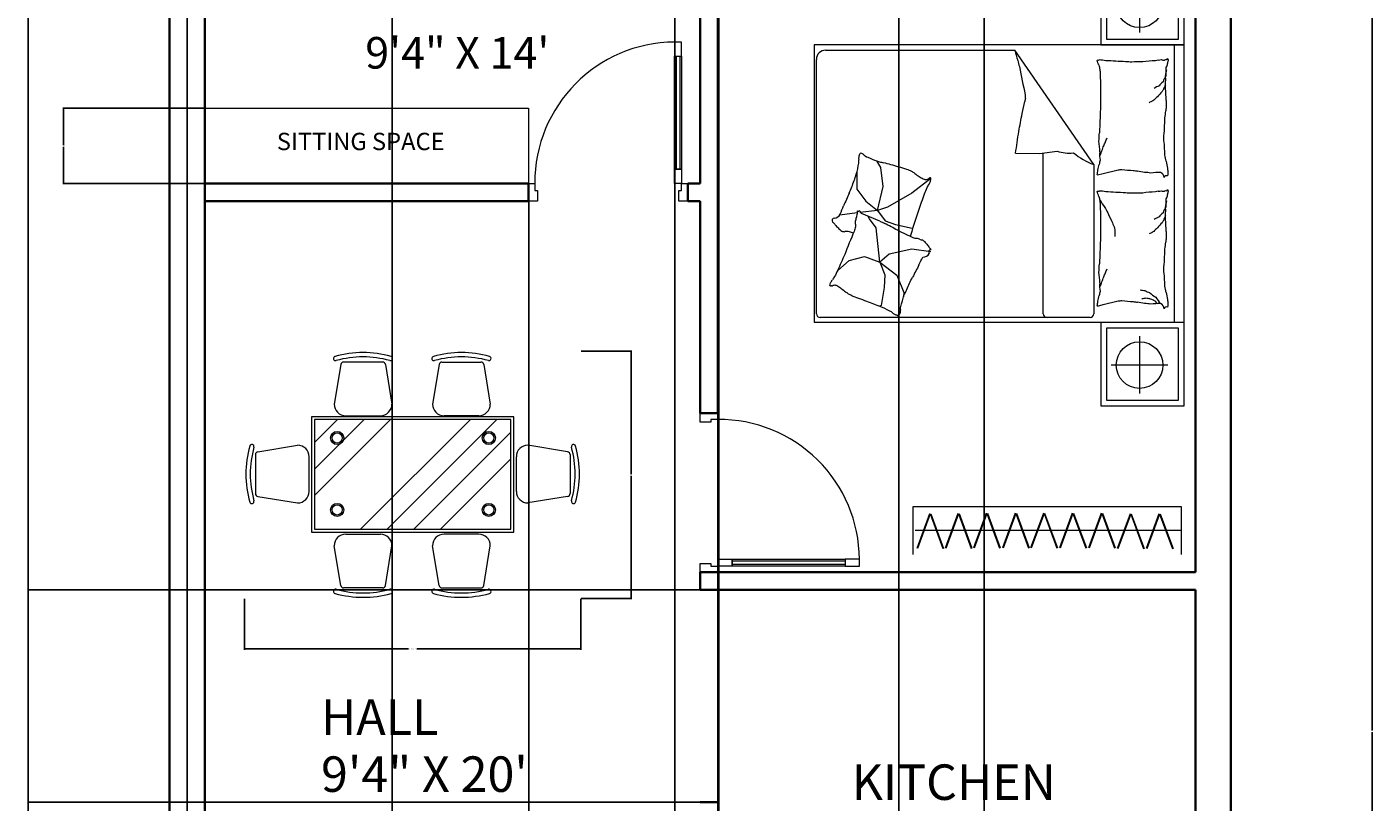
# Model space of a CAD drawing. Units: feet. Extents: x 1993 to 2298, y 2938 to 3641.
# Tile 8 of 11: x 1993 to 2298, y 3293 to 3468. Entities that reach past the tile are written whole.
import ezdxf

# ---------------------------------------------------------------- set-up
doc = ezdxf.new("R2010")
doc.units = ezdxf.units.FT
for name, color, linetype, lineweight in [('A-ANNO-DIMS', 2, 'Continuous', 18), ('A-AREA-IDEN', 7, 'Continuous', 18), ('A-DOOR', 3, 'Continuous', 18), ('A-FLOR-CASE', 8, 'Continuous', 18), ('furniture', 8, 'Continuous', 18), ('WAL', 7, 'Continuous', 35), ('wardrobe', 4, 'Continuous', 13)]:
    doc.layers.add(name, color=color, linetype=linetype, lineweight=lineweight)
doc.styles.add('DIM_FONT', font='SIMPLEX.shx', dxfattribs={"width": 0.8})
doc.styles.get("Standard").update_dxf_attribs({"font": 'arial.ttf'})
doc.dimstyles.get("Standard").update_dxf_attribs({"dimtxt": 0.18, "dimasz": 0.18, "dimexe": 0.18, "dimexo": 0.0625, "dimgap": 0.09, "dimtad": 0, "dimtih": 1, "dimtoh": 1, "dimdec": 4, "dimzin": 0, "dimdsep": 46, "dimtxsty": 'Standard', "dimcen": 0.09, "dimadec": 0, "dimazin": 0, "dimtfac": 1, "dimtdec": 4, "dimtofl": 0, "dimtmove": 0, "dimatfit": 3, "dimfxl": 1, "dimtolj": 1, "dimtzin": 0, "dimarcsym": 0})

# ---------------------------------------------------------------- blocks, each defined once
blk = doc.blocks.new('A$C184E58E8')
for points in [[(825, 900), (825, 820), (865, 820), (865, 900)], [(825, 180), (825, 820), (865, 820), (865, 180)], [(835, 180), (835, 820), (855, 820), (855, 180)], [(825, 100), (825, 180), (865, 180), (865, 100)], [(35, 100), (35, 60), (50, 60), (50, 50), (50, 0), (0, 0), (0, 100)], [(865, 100), (900, 100), (900, 0), (850, 0), (850, 50), (850, 60), (865, 60)]]:
    blk.add_lwpolyline(points, close=True)
blk.add_arc((830, 105), 795, 90.36035, 180.36035)
blk = doc.blocks.new('A$C79766A75')
for p, q in [((0.45, 1.9999), (0, 1.9999)), ((0, 1.9999), (0, 1.5499)), ((0.42, 1.9699), (0.03, 1.9699)), ((0.03, 1.9699), (0.03, 1.5799)), ((0.42, 1.5799), (0.42, 1.9699)), ((0.45, 1.5499), (0.45, 1.9999)), ((1.9506, 2), (0.4506, 2)), ((0.4506, 2), (0.4506, 0)), ((1.9506, 0), (1.9506, 2)), ((2.402, 1.9999), (1.952, 1.9999)), ((1.952, 1.9999), (1.952, 1.5499)), ((2.372, 1.9699), (1.982, 1.9699)), ((1.982, 1.9699), (1.982, 1.5799)), ((2.372, 1.5799), (2.372, 1.9699)), ((2.402, 1.5499), (2.402, 1.9999)), ((0.2304, 1.9125), (0.2304, 1.6061)), ((1.9506, 1.9476), (0.4506, 1.9476)), ((2.1824, 1.9125), (2.1824, 1.6061)), ((0.0743, 1.7595), (0.3834, 1.7595)), ((2.0263, 1.7595), (2.3354, 1.7595)), ((0.4234, 1.6034), (0.4228, 1.6034)), ((1.1461, 1.5617), (1.1254, 1.6443)), ((1.8553, 1.5617), (1.8346, 1.6443)), ((0, 1.5499), (0.45, 1.5499)), ((0.03, 1.5799), (0.42, 1.5799)), ((1.1536, 1.5317), (1.1461, 1.5617)), ((1.8628, 1.5317), (1.8553, 1.5617)), ((1.952, 1.5499), (2.402, 1.5499)), ((1.982, 1.5799), (2.372, 1.5799)), ((1.0972, 1.5115), (0.4791, 1.0841)), ((1.0972, 1.5115), (1.9048, 1.5115)), ((1.9248, 1.4915), (1.9248, 0.0322)), ((1.0383, 1.2184), (1.0246, 1.3138)), ((1.9048, 1.2389), (1.0354, 1.2389)), ((1.0365, 1.0883), (1.0383, 1.2184)), ((0.4791, 0.0622), (0.4791, 1.0841)), ((1.1731, 0.6316), (1.2523, 0.5276)), ((1.5696, 0.6317), (1.5559, 0.5286)), ((1.2523, 0.5276), (1.3274, 0.3973)), ((1.4223, 0.4407), (1.442, 0.5296)), ((1.5559, 0.5286), (1.5817, 0.4065)), ((1.4025, 0.3834), (1.4223, 0.4407)), ((1.6264, 0.355), (1.6952, 0.4478)), ((1.6952, 0.4478), (1.7898, 0.4856)), ((1.7898, 0.4856), (1.8139, 0.4822)), ((1.2167, 0.3736), (1.1139, 0.3597)), ((1.3452, 0.342), (1.2167, 0.3736)), ((1.3274, 0.3973), (1.3452, 0.342)), ((1.3452, 0.342), (1.4025, 0.3834)), ((1.5817, 0.4065), (1.6264, 0.355)), ((1.6264, 0.355), (1.6935, 0.3825)), ((1.6935, 0.3825), (1.7623, 0.379)), ((1.7623, 0.379), (1.8603, 0.3619)), ((1.1139, 0.3597), (1.0779, 0.3397)), ((1.2957, 0.2787), (1.3452, 0.342)), ((1.3452, 0.342), (1.3569, 0.2478)), ((1.3803, 0.2995), (1.3626, 0.256)), ((1.3907, 0.3), (1.3787, 0.2914)), ((1.4034, 0.3558), (1.3803, 0.2995)), ((1.4406, 0.3361), (1.3907, 0.3)), ((1.6264, 0.355), (1.4406, 0.3361)), ((1.5954, 0.2725), (1.6264, 0.355)), ((1.8603, 0.3619), (1.8636, 0.3554)), ((1.1376, 0.2313), (1.2305, 0.2313)), ((1.2305, 0.2313), (1.2957, 0.2787)), ((1.3588, 0.2331), (1.3706, 0.1385)), ((1.6161, 0.19), (1.5954, 0.2725)), ((1.6697, 0.1274), (1.6161, 0.19)), ((1.9048, 0.0122), (0.5291, 0.0122)), ((0.4506, 0), (1.9506, 0))]:
    blk.add_line(p, q)
for centre in [(0.2304, 1.7595), (2.1824, 1.7595)]:
    blk.add_circle(centre, 0.126)
for centre, radius, start, end in [((0.5232, 1.9139), 0.00342, 291.7883, 340.43603), ((0.525, 1.9085), 0.00232, 340.43603, 101.89306), ((0.5246, 1.9378), 0.0251, 274.30254, 291.7883), ((0.5311, 1.9093), 0.00428, 201.9904, 281.89306), ((0.4996, 1.8889), 0.0328, 338.57902, 8.13348), ((0.5465, 1.8994), 0.0156, 158.57902, 201.9904), ((0.5486, 1.9393), 0.0289, 239.34875, 274.30254), ((0.5458, 1.8568), 0.0539, 59.34875, 84.74081), ((0.546, 1.0829), 0.8208, 84.74081, 88.09211), ((0.6118, 2.0005), 0.0992, 254.06476, 274.21588), ((0.6775, 1.9817), 0.0992, 233.91364, 254.06476), ((0.6362, 0.406), 1.4943, 88.09211, 90.57574), ((0.7737, 2.1075), 0.234, 242.76041, 249.13972), ((0.7591, 1.0293), 0.8732, 90.57574, 94.80185), ((0.7631, 2.1919), 0.2897, 267.46141, 274.80185), ((0.8143, 2.0532), 0.1524, 259.81012, 267.46141), ((0.7515, 1.3747), 0.5293, 79.81012, 83.9133), ((0.8451, 0.8466), 1.049, 83.9133, 90), ((1.046, 1.2129), 0.6827, 90, 97.54685), ((1.1117, 1.6625), 0.2422, 97.54685, 105.74398), ((1.0352, 2.2041), 0.3048, 278.43719, 285.74398), ((1.1179, 2.0719), 0.1611, 270, 278.43719), ((1.171, 1.8579), 0.0342, 94.40021, 153.41948), ((1.1592, 2.0011), 0.0904, 258.72762, 270), ((1.1709, 1.9049), 0.0131, 153.41948, 258.72762), ((1.2325, 1.9139), 0.00342, 291.7883, 340.43603), ((1.2342, 1.9085), 0.00232, 340.43603, 101.89306), ((1.2338, 1.9378), 0.0251, 274.30254, 291.7883), ((1.2404, 1.9093), 0.00428, 201.9904, 281.89306), ((1.2088, 1.8889), 0.0328, 338.57902, 8.13348), ((1.2558, 1.8994), 0.0156, 158.57902, 201.9904), ((1.2578, 1.9393), 0.0289, 239.34875, 274.30254), ((1.2551, 1.8568), 0.0539, 59.34875, 84.74081), ((1.2552, 1.0829), 0.8208, 84.74081, 88.09211), ((1.3211, 2.0005), 0.0992, 254.06476, 274.21588), ((1.3868, 1.9817), 0.0992, 233.91364, 254.06476), ((1.3455, 0.406), 1.4943, 88.09211, 90.57574), ((1.4829, 2.1075), 0.234, 242.76041, 249.13972), ((1.4683, 1.0293), 0.8732, 90.57574, 94.80185), ((1.4724, 2.1919), 0.2897, 267.46141, 274.80185), ((1.5236, 2.0532), 0.1524, 259.81012, 267.46141), ((1.4607, 1.3747), 0.5293, 79.81012, 83.9133), ((1.5543, 0.8466), 1.049, 83.9133, 90), ((1.7552, 1.2129), 0.6827, 90, 97.54685), ((1.821, 1.6625), 0.2422, 97.54685, 105.74398), ((1.7444, 2.2041), 0.3048, 278.43719, 285.74398), ((1.8271, 2.0719), 0.1611, 270, 278.43719), ((1.8802, 1.8579), 0.0342, 94.40021, 153.41948), ((1.8684, 2.0011), 0.0904, 258.72762, 270), ((1.8802, 1.9049), 0.0131, 153.41948, 258.72762), ((0.2896, 1.8253), 0.246, 8.13348, 12.10946), ((0.7297, 1.8867), 0.1983, 187.6809, 192.10946), ((1.4472, 1.8987), 0.9131, 183.36875, 187.6809), ((0.7304, 1.9449), 0.0992, 216.17665, 233.91364), ((0.7661, 1.8961), 0.0992, 198.43965, 216.17665), ((0.738, 1.949), 0.0768, 231.61143, 242.76041), ((0.974, 2.1633), 0.3916, 226.18849, 231.61143), ((0.9057, 1.9982), 0.2252, 219.03494, 226.18849), ((0.7932, 1.8591), 0.0493, 208.31676, 219.03494), ((0.9392, 1.9062), 0.2002, 203.00277, 208.31676), ((1.6324, 1.8735), 0.4918, 180, 186.23236), ((1.3446, 1.7858), 0.204, 170.31563, 180), ((0.9988, 1.8253), 0.246, 8.13348, 12.10946), ((1.4389, 1.8867), 0.1983, 187.6809, 192.10946), ((2.1565, 1.8987), 0.9131, 183.36875, 187.6809), ((1.4396, 1.9449), 0.0992, 216.17665, 233.91364), ((1.4753, 1.8961), 0.0992, 198.43965, 216.17665), ((1.4473, 1.949), 0.0768, 231.61143, 242.76041), ((1.6833, 2.1633), 0.3916, 226.18849, 231.61143), ((1.615, 1.9982), 0.2252, 219.03494, 226.18849), ((1.5025, 1.8591), 0.0493, 208.31676, 219.03494), ((1.6484, 1.9062), 0.2002, 203.00277, 208.31676), ((1.6908, 1.9123), 0.1399, 314.90238, 332.60117), ((1.7511, 1.9723), 0.1399, 297.20359, 314.90238), ((1.6307, 1.8895), 0.2056, 338.18508, 341.2201), ((1.6887, 1.8881), 0.1511, 334.64488, 338.18508), ((1.7896, 1.8667), 0.0526, 318.55709, 334.64488), ((1.784, 1.9167), 0.0899, 306.26407, 318.55709), ((2.3416, 1.8735), 0.4918, 180, 186.23236), ((2.0538, 1.7858), 0.204, 170.31563, 180), ((1.2208, 1.7573), 0.6787, 178.36691, 183.36875), ((0.8192, 1.792), 0.3171, 347.80162, 351.99495), ((2.0027, 1.5994), 0.882, 167.80162, 170.31563), ((1.9301, 1.7573), 0.6787, 178.36691, 183.36875), ((1.6404, 1.8023), 0.1399, 343.48502, 354.36887), ((1.6554, 1.8529), 0.1399, 332.60117, 343.48502), ((1.7653, 1.8132), 0.0562, 341.2201, 0), ((1.73, 1.7719), 0.0915, 0, 14.68511), ((1.5284, 1.792), 0.3171, 347.80162, 351.99495), ((2.7119, 1.5994), 0.882, 167.80162, 170.31563), ((14.1519, 0.85), 13.6356, 176.49514, 176.94504), ((1.9066, 1.6447), 1.3652, 176.94504, 178.36691), ((0.4711, 1.7556), 0.6588, 351.99495, 357.33512), ((14.8612, 0.85), 13.6356, 176.49514, 176.94504), ((2.6158, 1.6447), 1.3652, 176.94504, 178.36691), ((1.1803, 1.7556), 0.6588, 351.99495, 357.33512), ((1.0578, 1.6474), 0.0677, 357.33512, 14.04519), ((0.7658, 2.8912), 1.4323, 294.32653, 296.49848), ((1.226, 2.0834), 0.5066, 290.67428, 294.32653), ((1.4305, 1.6796), 0.058, 274.08277, 290.67428), ((1.4679, 1.8969), 0.2721, 266.4448, 274.08277), ((1.767, 1.6474), 0.0677, 357.33512, 14.04519), ((0.8521, 1.5209), 0.3212, 170.00164, 176.49514), ((0.513, 1.535), 0.0193, 350.00164, 16.69777), ((0.5322, 1.5304), 0.00132, 16.69777, 97.12039), ((0.5579, 1.4467), 0.0875, 97.12039, 106.22115), ((0.5822, 1.4654), 0.0767, 106.22115, 117.28412), ((0.5507, 1.5832), 0.0453, 282.86904, 297.28412), ((0.5623, 1.6885), 0.1459, 273.57397, 282.86904), ((0.589, 2.7103), 1.164, 270.28654, 273.57397), ((0.7584, 7.2662), 5.7185, 269.02962, 270.28654), ((0.9401, 4.9065), 3.3622, 267.39037, 269.02962), ((0.9811, 2.7573), 1.2165, 265.38242, 267.39037), ((0.8583, 0.139), 1.4048, 85.38242, 87.25094), ((0.6583, 0.9067), 0.7387, 64.68893, 66.51559), ((1.0175, 1.3138), 0.2301, 87.25094, 101.55856), ((0.7015, 0.888), 0.7387, 66.51559, 68.34226), ((0.7501, 0.8688), 0.7387, 68.34226, 70.57202), ((0.8043, 0.8497), 0.7387, 70.57202, 72.80178), ((1.0449, 1.6886), 0.1459, 263.56595, 281.55856), ((1.1099, 1.6599), 0.1197, 252.61359, 263.56595), ((1.0587, 1.3144), 0.2297, 72.61359, 80.5159), ((1.108, 1.2635), 0.2708, 80.5159, 85.91706), ((1.1535, 1.5308), 0.000917, 85.91706, 194.04494), ((1.5613, 1.5209), 0.3212, 170.00164, 176.49514), ((1.2222, 1.535), 0.0193, 350.00164, 16.69777), ((1.2414, 1.5304), 0.00132, 16.69777, 97.12039), ((1.2671, 1.4467), 0.0875, 97.12039, 106.22115), ((1.2914, 1.4654), 0.0767, 106.22115, 117.28412), ((1.2599, 1.5832), 0.0453, 282.86904, 297.28412), ((1.2716, 1.6885), 0.1459, 273.57397, 282.86904), ((0.9025, 2.1618), 0.7286, 302.13498, 305.82629), ((1.2982, 2.7103), 1.164, 270.28654, 273.57397), ((1.1895, 1.8508), 0.3126, 296.49848, 302.13498), ((1.4677, 7.2662), 5.7185, 269.02962, 270.28654), ((1.6493, 4.9065), 3.3622, 267.39037, 269.02962), ((1.6903, 2.7573), 1.2165, 265.38242, 267.39037), ((1.5676, 0.139), 1.4048, 85.38242, 87.25094), ((1.3675, 0.9067), 0.7387, 64.68893, 66.51559), ((1.7268, 1.3138), 0.2301, 87.25094, 101.55856), ((1.4107, 0.888), 0.7387, 66.51559, 68.34226), ((1.4594, 0.8688), 0.7387, 68.34226, 70.57202), ((1.5136, 0.8497), 0.7387, 70.57202, 72.80178), ((1.7541, 1.6886), 0.1459, 263.56595, 281.55856), ((1.8192, 1.6599), 0.1197, 252.61359, 263.56595), ((1.7679, 1.3144), 0.2297, 72.61359, 80.5159), ((1.8172, 1.2635), 0.2708, 80.5159, 85.91706), ((1.8627, 1.5308), 0.000917, 85.91706, 194.04494), ((0.745, 1.6407), 0.3751, 320.35546, 339.85116), ((1.9048, 1.4915), 0.02, 0, 90), ((0.8556, 1.3759), 0.1801, 339.85116, 8.13558), ((1.9048, 1.2589), 0.02, 270, 0), ((-0.0248, 2.8487), 1.8351, 285.93519, 287.73639), ((0.3872, 1.7415), 0.6574, 282.92554, 285.93519), ((-0.1888, 5.1029), 4.0646, 280.72756, 282.92554), ((0.7282, 1.1989), 0.0581, 262.26962, 280.72756), ((0.7833, 1.3309), 0.1942, 256.8096, 262.26962), ((0.2481, -1.3253), 2.5158, 76.8096, 78.32586), ((0.3953, -1.4284), 2.588, 78.32586, 80.50498), ((0.413, -2.64), 3.7801, 80.50498, 82.308), ((0.8605, 0.749), 0.352, 329.09437, 333.18207), ((1.1752, 0.6267), 0.0063, 166.71916, 233.42082), ((1.1734, 0.6272), 0.00443, 93.94836, 166.71916), ((1.163, 0.6103), 0.0142, 10.40739, 53.42082), ((1.1755, 0.5964), 0.0352, 69.65479, 93.94836), ((1.1396, 0.6079), 0.0393, 333.18207, 345.42909), ((1.1011, 0.5989), 0.0771, 2.72862, 10.40739), ((1.1628, 0.6019), 0.0153, 345.42909, 2.72862), ((1.1669, 0.5731), 0.0601, 51.41461, 69.65479), ((1.2538, 0.682), 0.0792, 231.41461, 247.29308), ((1.5463, 1.3811), 0.8371, 247.29308, 249.87133), ((3.0113, 5.3783), 5.0942, 249.87133, 250.91638), ((1.4828, 0.5833), 0.0226, 324.10643, 8.04918), ((1.4519, 0.6426), 0.0774, 313.52244, 324.10643), ((1.383, 0.7705), 0.2176, 307.21509, 313.52244), ((1.1426, 1.1456), 0.6605, 306.2163, 307.21509), ((1.7751, 0.3162), 0.3825, 126.2163, 127.52874), ((1.5806, 0.5924), 0.0452, 127.52874, 134.1274), ((1.5093, 0.6825), 0.0697, 308.81361, 314.1274), ((1.5706, 0.6318), 0.0127, 176.75451, 308.81361), ((1.5621, 0.59), 0.0359, 356.75451, 62.70976), ((0.2201, -2.1858), 3.0972, 62.70976, 63.58535), ((1.3115, 0.4414), 0.1965, 153.92651, 162.1604), ((1.2077, 0.4922), 0.081, 140.29953, 153.92651), ((0.9961, 0.6678), 0.194, 320.29953, 329.09437), ((2.374, 3.5362), 3.145, 250.91638, 253.39153), ((1.5084, 0.6341), 0.1166, 253.39153, 259.26338), ((2.4089, 0.1204), 1.0054, 154.94715, 157.58378), ((1.5435, 0.5526), 0.0458, 157.58378, 188.04918), ((2.5711, 2.3551), 2.0162, 242.50014, 243.58535), ((4.5245, 5.9445), 6.1019, 242.15178, 242.50014), ((-0.9881, -4.647), 5.8383, 62.15178, 62.50792), ((1.5182, -0.068), 0.6236, 62.50792, 69.25137), ((3.0311, -0.112), 2.003, 162.1604, 164.73746), ((2.8096, -0.3311), 1.5652, 150.06403, 152.91165), ((2.9813, -0.2643), 1.6868, 152.91165, 154.94715), ((1.7121, 0.0657), 0.43, 69.25137, 77.37478), ((1.8682, 0.4049), 0.063, 77.37478, 93.38812), ((1.8955, 0.5247), 0.0599, 256.95977, 273.38812), ((1.8435, 0.4743), 0.0755, 310.50865, 333.66682), ((1.9257, 0.5082), 0.0509, 238.30826, 256.95977), ((1.9279, 0.441), 0.0168, 130.50865, 180.96136), ((1.9201, 0.4587), 0.0058, 180.96136, 238.30826), ((0.5589, 0.5062), 0.5454, 343.68776, 346.159), ((2.6887, -0.0186), 1.6481, 164.73746, 166.159), ((1.2176, 0.4627), 0.2143, 330.06403, 337.76452), ((1.701, 0.4319), 0.1798, 334.82685, 339.29188), ((-0.5166, 1.5491), 2.6619, 333.66682, 334.82685), ((-1.4109, 1.284), 2.6619, 338.0627, 339.22273), ((0.9098, 0.4035), 0.1798, 339.22273, 343.68776), ((3.6966, -0.4634), 2.003, 157.76452, 160.34158), ((3.4079, -0.2212), 1.6481, 160.34158, 161.76311), ((1.3456, 0.5261), 0.5454, 339.29188, 341.76311), ((1.0533, 0.2524), 0.0168, 134.90453, 185.35724), ((1.0424, 0.2513), 0.0058, 185.35724, 242.70414), ((1.0631, 0.2914), 0.0509, 242.70414, 261.35565), ((0.9882, 0.3177), 0.0755, 314.90453, 338.0627), ((1.0645, 0.3003), 0.0599, 261.35565, 277.784), ((1.0811, 0.1786), 0.063, 81.77066, 97.784), ((1.0286, -0.1846), 0.43, 73.64725, 81.77066), ((0.974, -0.3705), 0.6236, 66.9038, 73.64725), ((1.3465, 0.2383), 0.00467, 287.18674, 70.62007), ((1.3486, 0.2247), 0.0092, 70.62007, 94.25932), ((1.3694, 0.234), 0.0231, 107.18674, 157.76452), ((1.3563, 0.267), 0.034, 262.01776, 274.25932), ((1.4091, 0.4221), 0.1955, 255.1193, 262.01776), ((1.358, 0.0507), 0.1794, 75.1193, 82.32164), ((1.4096, 0.153), 0.0712, 82.32164, 94.51184), ((1.4285, 0.2893), 0.0663, 261.87843, 274.51184), ((1.4755, 0.332), 0.1166, 248.99565, 261.87843), ((-1.0716, -5.1672), 5.8383, 66.54766, 66.9038), ((3.6805, 5.7866), 6.1019, 246.54766, 246.89602), ((2.0773, 2.0287), 2.0162, 246.89602, 247.98123), ((0.1602, -2.7118), 3.0972, 67.10564, 67.98123), ((1.3914, 0.1905), 0.0774, 317.91833, 328.50231), ((1.4382, 0.1619), 0.0226, 328.50231, 12.44506), ((2.7121, 3.1012), 3.145, 246.5205, 248.99565), ((1.505, 0.1766), 0.0458, 161.97966, 192.44506), ((2.4175, -0.1202), 1.0054, 160.65521, 161.97966), ((3.6993, 4.7998), 5.0942, 245.47545, 246.5205), ((1.4661, 0.3294), 0.352, 324.69849, 328.78619), ((1.6279, 0.2819), 0.194, 315.90365, 324.69849), ((1.856, 0.1288), 0.081, 135.90365, 149.53063), ((1.9797, 0.1108), 0.1965, 149.53063, 157.76452), ((1.3512, 0.1084), 0.0359, 1.15039, 67.10564), ((1.3997, 0.1094), 0.0127, 181.15039, 313.2095), ((1.3607, 0.1509), 0.0697, 313.2095, 318.52329), ((1.4468, 0.0748), 0.0452, 131.92462, 138.52329), ((1.6722, -0.1762), 0.3825, 130.61218, 131.92462), ((0.9933, 0.6156), 0.6605, 310.61218, 311.61098), ((1.2874, 0.2845), 0.2176, 311.61098, 317.91833), ((2.051, 0.8725), 0.8371, 242.8972, 245.47545), ((1.7576, 0.1689), 0.0792, 227.01873, 242.8972), ((1.6963, 0.0438), 0.0601, 47.01873, 65.25891), ((1.737, 0.0526), 0.0352, 65.25891, 89.55248), ((1.7345, 0.1188), 0.0153, 341.03321, 358.33274), ((1.6723, 0.1058), 0.0771, 358.33274, 6.01151), ((1.7401, 0.0928), 0.0142, 6.01151, 49.02494), ((1.7162, 0.1388), 0.0393, 328.78619, 341.03321), ((1.756, 0.0832), 0.00443, 89.55248, 162.32327), ((1.7602, 0.0924), 0.0063, 162.32327, 229.02494), ((0.5291, 0.0622), 0.05, 180, 270), ((1.9048, 0.0322), 0.02, 270, 0)]:
    blk.add_arc(centre, radius, start, end)
at = {"style": 'DIM_FONT', "text_generation_flag": 4, "width": 0.8, "flags": 9}
for tag in ['XSIZE', 'YSIZE']:
    blk.add_attdef(tag, (1.9506, 2), '', height=0.0005, rotation=180, dxfattribs=at)
blk = doc.blocks.new('A$C199426D1')
for p, q in [((-208.8, 378.9), (-478.9, 378.9)), ((202.6, 378.9), (472.7, 378.9)), ((-498.7, 362.2), (-543.8, 87.1)), ((-189, 362.2), (-143.8, 87.1)), ((182.8, 362.2), (137.6, 87.1)), ((492.5, 362.2), (537.6, 87.1)), ((-700, 0), (-700, -800)), ((700, 0), (-700, 0)), ((-463.8, 7.1), (-223.8, 7.1)), ((457.6, 7.1), (217.6, 7.1)), ((700, -800), (700, 0)), ((-680, -178.8), (-521.2, -20)), ((-680, -20), (-680, -780)), ((-680, -547), (-153, -20)), ((680, -20), (-680, -20)), ((-481.1, -164), (-337.1, -20)), ((-360.7, -780), (399.3, -20)), ((-176.6, -780), (583.4, -20)), ((680, -780), (680, -20)), ((7.4, -780), (680, -107.4)), ((-1089.5, -262.3), (-1089.5, -532.5)), ((-1072.8, -242.6), (-797.7, -197.4)), ((-717.7, -517.4), (-717.7, -277.4)), ((-680, -362.9), (-506.9, -189.8)), ((717.7, -517.4), (717.7, -277.4)), ((1072.8, -242.6), (797.7, -197.4)), ((1089.5, -262.3), (1089.5, -532.5)), ((191.5, -780), (680, -291.5)), ((-1072.8, -552.3), (-797.7, -597.4)), ((1072.8, -552.3), (797.7, -597.4)), ((-700, -800), (700, -800)), ((-680, -780), (680, -780)), ((-463.8, -814.1), (-223.8, -814.1)), ((457.6, -814.1), (217.6, -814.1)), ((-498.7, -1169.2), (-543.8, -894.1)), ((-189, -1169.2), (-143.8, -894.1)), ((182.8, -1169.2), (137.6, -894.1)), ((492.5, -1169.2), (537.6, -894.1)), ((-208.8, -1185.9), (-478.9, -1185.9)), ((202.6, -1185.9), (472.7, -1185.9))]:
    blk.add_line(p, q)
for centre, radius in [((-523.4, -147.5), 45.4), ((-523.4, -147.5), 35.4), ((527, -147.5), 45.4), ((527, -147.5), 35.4), ((-523.4, -646), 45.4), ((-523.4, -646), 35.4), ((527, -646), 45.4), ((527, -646), 35.4)]:
    blk.add_circle(centre, radius)
for centre, radius, start, end in [((-533.8, 403.4), 15, 105.49005, 284.28424), ((-343.8, -280), 724.3, 74.47014, 105.57697), ((-343.8, -279.6), 693.9, 74.43245, 105.56755), ((-478.9, 358.9), 20, 90, 170.67171), ((-208.8, 358.9), 20, 9.32829, 90), ((-153.9, 403.4), 15, 255.71576, 74.50995), ((147.7, 403.4), 15, 105.49005, 284.28424), ((337.6, -280), 724.3, 74.42303, 105.52986), ((337.6, -279.6), 693.9, 74.43245, 105.56755), ((202.6, 358.9), 20, 90, 170.67171), ((472.7, 358.9), 20, 9.32829, 90), ((527.6, 403.4), 15, 255.71576, 74.50995), ((-463.8, 87.1), 80, 180, 270), ((-223.8, 87.1), 80, 270, 0), ((217.6, 87.1), 80, 180, 270), ((457.6, 87.1), 80, 270, 0), ((-430.6, -397.4), 724.3, 164.47014, 195.57697), ((-1113.9, -207.5), 15, 345.71576, 164.50995), ((-430.9, -397.4), 693.9, 164.43245, 195.56755), ((-1069.5, -262.3), 20, 99.32829, 180), ((-797.7, -277.4), 80, 0, 90), ((797.7, -277.4), 80, 90, 180), ((1069.5, -262.3), 20, 0, 80.67171), ((1113.9, -207.5), 15, 15.49005, 194.28424), ((430.9, -397.4), 693.9, 344.43245, 15.56755), ((430.6, -397.4), 724.3, 344.42303, 15.52986), ((-1069.5, -532.5), 20, 180, 260.67171), ((-797.7, -517.4), 80, 270, 0), ((797.7, -517.4), 80, 180, 270), ((1069.5, -532.5), 20, 279.32829, 0), ((-1113.9, -587.4), 15, 195.49005, 14.28424), ((1113.9, -587.4), 15, 165.71576, 344.50995), ((-463.8, -894.1), 80, 90, 180), ((-223.8, -894.1), 80, 0, 90), ((217.6, -894.1), 80, 90, 180), ((457.6, -894.1), 80, 0, 90), ((-533.8, -1210.3), 15, 75.71576, 254.50995), ((-343.8, -527.3), 693.9, 254.43245, 285.56755), ((-478.9, -1165.9), 20, 189.32829, 270), ((-208.8, -1165.9), 20, 270, 350.67171), ((-153.9, -1210.3), 15, 285.49005, 104.28424), ((147.7, -1210.3), 15, 75.71576, 254.50995), ((337.6, -527.3), 693.9, 254.43245, 285.56755), ((202.6, -1165.9), 20, 189.32829, 270), ((472.7, -1165.9), 20, 270, 350.67171), ((527.6, -1210.3), 15, 285.49005, 104.28424), ((-343.8, -527), 724.3, 254.42303, 285.52986), ((337.6, -527), 724.3, 254.47014, 285.57697)]:
    blk.add_arc(centre, radius, start, end)
blk = doc.blocks.new('WARDROBE-PLAN')
for p, q in [((4.82, 1.61), (1.93, 9.47)), ((4.96, 1.67), (2.08, 9.52)), ((4.96, 1.67), (7.85, 9.52)), ((5.11, 1.61), (7.99, 9.46)), ((11.37, 1.61), (8.49, 9.46)), ((11.51, 1.67), (8.63, 9.52)), ((11.51, 1.67), (14.4, 9.52)), ((11.66, 1.61), (14.54, 9.46)), ((17.87, 1.47), (14.98, 9.32)), ((18.01, 1.52), (15.13, 9.37)), ((18.01, 1.52), (20.9, 9.37)), ((18.16, 1.47), (21.04, 9.32)), ((24.42, 1.47), (21.53, 9.32)), ((24.56, 1.52), (21.68, 9.37)), ((24.56, 1.52), (27.45, 9.37)), ((24.71, 1.47), (27.59, 9.32)), ((30.97, 1.47), (28.09, 9.32)), ((31.11, 1.52), (28.23, 9.37)), ((31.11, 1.52), (34, 9.37)), ((31.26, 1.47), (34.14, 9.32)), ((37.35, 1.47), (34.47, 9.32)), ((37.5, 1.52), (34.62, 9.37)), ((37.5, 1.52), (40.38, 9.37)), ((37.64, 1.47), (40.53, 9.32)), ((43.9, 1.46), (41.02, 9.32)), ((44.05, 1.52), (41.17, 9.37)), ((44.05, 1.52), (46.93, 9.37)), ((44.19, 1.46), (47.08, 9.32)), ((50.31, 1.52), (47.43, 9.37)), ((50.46, 1.57), (47.57, 9.42)), ((50.46, 1.57), (53.34, 9.42)), ((50.6, 1.52), (53.49, 9.37)), ((56.72, 1.57), (53.83, 9.42)), ((56.86, 1.62), (53.98, 9.47)), ((56.86, 1.62), (59.75, 9.47)), ((57.01, 1.57), (59.89, 9.42)), ((0, 5.4), (60.23, 5.39))]:
    blk.add_line(p, q)
blk.add_lwpolyline([(0, 10.78), (0, 0.01), (60.75, 0), (60.75, 10.78)])
blk = doc.blocks.new('*D40')
at = {"layer": 'A-ANNO-DIMS', "color": 0, "lineweight": -2, "transparency": 16777216}
for p, q in [((2042.73, 3338.53), (2042.73, 3327.01)), ((2118.74, 3338.53), (2118.74, 3327.01)), ((2042.91, 3327.19), (2079.76, 3327.19)), ((2118.56, 3327.19), (2081.7, 3327.19))]:
    blk.add_line(p, q, dxfattribs=at)
at = {"layer": 'A-ANNO-DIMS', "color": 0, "transparency": 16777216}
for points in [[(2042.91, 3327.22), (2042.91, 3327.16), (2042.73, 3327.19)], [(2118.56, 3327.22), (2118.56, 3327.16), (2118.74, 3327.19)]]:
    blk.add_solid(points, dxfattribs=at)
at = {"layer": 'Defpoints', "color": 0, "transparency": 16777216}
for p in [(2042.73, 3338.59), (2118.74, 3338.59), (2118.74, 3327.19)]:
    blk.add_point(p, dxfattribs=at)
at = {"layer": 'A-ANNO-DIMS', "color": 0, "transparency": 16777216, "insert": (2080.73, 3327.19), "char_height": 0.18, "attachment_point": 5}
blk.add_mtext('\\A1;DINING SET 76', dxfattribs=at)
blk = doc.blocks.new('*D41')
at = {"layer": 'A-ANNO-DIMS', "color": 0, "lineweight": -2, "transparency": 16777216}
for p, q in [((2118.8, 3394.54), (2130.32, 3394.54)), ((2130.14, 3394.36), (2130.14, 3366.75)), ((2130.14, 3338.77), (2130.14, 3366.39)), ((2118.8, 3338.59), (2130.32, 3338.59))]:
    blk.add_line(p, q, dxfattribs=at)
at = {"layer": 'A-ANNO-DIMS', "color": 0, "transparency": 16777216}
for points in [[(2130.11, 3394.36), (2130.17, 3394.36), (2130.14, 3394.54)], [(2130.11, 3338.77), (2130.17, 3338.77), (2130.14, 3338.59)]]:
    blk.add_solid(points, dxfattribs=at)
at = {"layer": 'Defpoints', "color": 0, "transparency": 16777216}
for p in [(2118.74, 3394.54), (2130.14, 3394.54), (2118.74, 3338.59)]:
    blk.add_point(p, dxfattribs=at)
at = {"layer": 'A-ANNO-DIMS', "color": 0, "transparency": 16777216, "insert": (2130.14, 3366.57), "char_height": 0.18, "attachment_point": 5}
blk.add_mtext('\\A1;56', dxfattribs=at)
blk = doc.blocks.new('*D55')
at = {"layer": 'A-ANNO-DIMS', "color": 0, "lineweight": -2, "transparency": 16777216}
for p, q in [((2265.82, 3608.53), (2297.9, 3608.53)), ((2297.72, 3608.35), (2297.72, 3308.72)), ((2297.72, 3008.71), (2297.72, 3308.35)), ((2265.82, 3008.53), (2297.9, 3008.53))]:
    blk.add_line(p, q, dxfattribs=at)
at = {"layer": 'A-ANNO-DIMS', "color": 0, "transparency": 16777216}
for points in [[(2297.69, 3608.35), (2297.75, 3608.35), (2297.72, 3608.53)], [(2297.69, 3008.71), (2297.75, 3008.71), (2297.72, 3008.53)]]:
    blk.add_solid(points, dxfattribs=at)
at = {"layer": 'Defpoints', "color": 0, "transparency": 16777216}
for p in [(2265.76, 3608.53), (2297.72, 3608.53), (2265.76, 3008.53)]:
    blk.add_point(p, dxfattribs=at)
at = {"layer": 'A-ANNO-DIMS', "color": 0, "transparency": 16777216, "insert": (2297.72, 3308.53), "char_height": 0.18, "attachment_point": 5}
blk.add_mtext('\\A1;600', dxfattribs=at)
blk = doc.blocks.new('*D56')
at = {"layer": 'A-ANNO-DIMS', "color": 0, "lineweight": -2, "transparency": 16777216}
for p, q in [((2025.7, 3608.53), (1993.61, 3608.53)), ((1993.79, 3608.35), (1993.79, 3289.45)), ((1993.79, 2970.18), (1993.79, 3289.08)), ((2029.7, 2970), (1993.61, 2970))]:
    blk.add_line(p, q, dxfattribs=at)
at = {"layer": 'A-ANNO-DIMS', "color": 0, "transparency": 16777216}
for points in [[(1993.76, 3608.35), (1993.82, 3608.35), (1993.79, 3608.53)], [(1993.76, 2970.18), (1993.82, 2970.18), (1993.79, 2970)]]:
    blk.add_solid(points, dxfattribs=at)
at = {"layer": 'Defpoints', "color": 0, "transparency": 16777216}
for p in [(1993.79, 3608.53), (2025.76, 3608.53), (2029.76, 2970)]:
    blk.add_point(p, dxfattribs=at)
at = {"layer": 'A-ANNO-DIMS', "color": 0, "transparency": 16777216, "insert": (1993.79, 3289.27), "char_height": 0.18, "attachment_point": 5}
blk.add_mtext('\\A1;638.5', dxfattribs=at)
blk = doc.blocks.new('*D59')
at = {"layer": 'A-ANNO-DIMS', "color": 0, "lineweight": -2, "transparency": 16777216}
for p, q in [((2140, 3048.6), (2140, 3640.68)), ((2140.18, 3640.5), (2144.79, 3640.5)), ((2149.82, 3640.5), (2145.21, 3640.5)), ((2150, 3048.6), (2150, 3640.68))]:
    blk.add_line(p, q, dxfattribs=at)
at = {"layer": 'A-ANNO-DIMS', "color": 0, "transparency": 16777216}
for points in [[(2140.18, 3640.53), (2140.18, 3640.47), (2140, 3640.5)], [(2149.82, 3640.53), (2149.82, 3640.47), (2150, 3640.5)]]:
    blk.add_solid(points, dxfattribs=at)
at = {"layer": 'Defpoints', "color": 0, "transparency": 16777216}
for p in [(2150, 3640.5), (2140, 3048.53), (2150, 3048.53)]:
    blk.add_point(p, dxfattribs=at)
at = {"layer": 'A-ANNO-DIMS', "color": 0, "transparency": 16777216, "insert": (2145, 3640.5), "char_height": 0.18, "attachment_point": 5}
blk.add_mtext('\\A1;10', dxfattribs=at)
blk = doc.blocks.new('*D62')
at = {"layer": 'A-ANNO-DIMS', "color": 0, "lineweight": -2, "transparency": 16777216}
for p, q in [((2145.7, 3340.53), (1993.61, 3340.53)), ((1993.79, 3340.35), (1993.79, 3316.72)), ((1993.79, 3292.71), (1993.79, 3316.35)), ((2145.7, 3292.53), (1993.61, 3292.53))]:
    blk.add_line(p, q, dxfattribs=at)
at = {"layer": 'A-ANNO-DIMS', "color": 0, "transparency": 16777216}
for points in [[(1993.76, 3340.35), (1993.82, 3340.35), (1993.79, 3340.53)], [(1993.76, 3292.71), (1993.82, 3292.71), (1993.79, 3292.53)]]:
    blk.add_solid(points, dxfattribs=at)
at = {"layer": 'Defpoints', "color": 0, "transparency": 16777216}
for p in [(1993.79, 3340.53), (2145.76, 3340.53), (2145.76, 3292.53)]:
    blk.add_point(p, dxfattribs=at)
at = {"layer": 'A-ANNO-DIMS', "color": 0, "transparency": 16777216, "insert": (1993.79, 3316.53), "char_height": 0.18, "attachment_point": 5}
blk.add_mtext('\\A1;48', dxfattribs=at)
blk = doc.blocks.new('*D67')
at = {"layer": 'A-ANNO-DIMS', "color": 0, "lineweight": -2, "transparency": 16777216}
for p, q in [((2033.76, 3428.47), (2033.76, 2937.86)), ((2106.96, 3428.47), (2106.96, 2937.86)), ((2033.94, 2938.03), (2070.03, 2938.03)), ((2106.78, 2938.03), (2070.68, 2938.03))]:
    blk.add_line(p, q, dxfattribs=at)
at = {"layer": 'A-ANNO-DIMS', "color": 0, "transparency": 16777216}
for points in [[(2033.94, 2938.07), (2033.94, 2938.01), (2033.76, 2938.03)], [(2106.78, 2938.07), (2106.78, 2938.01), (2106.96, 2938.03)]]:
    blk.add_solid(points, dxfattribs=at)
at = {"layer": 'Defpoints', "color": 0, "transparency": 16777216}
for p in [(2033.76, 3428.53), (2106.96, 3428.53), (2106.96, 2938.03)]:
    blk.add_point(p, dxfattribs=at)
at = {"layer": 'A-ANNO-DIMS', "color": 0, "transparency": 16777216, "insert": (2070.36, 2938.03), "char_height": 0.18, "attachment_point": 5}
blk.add_mtext('\\A1;73.2', dxfattribs=at)
blk = doc.blocks.new('*D68')
at = {"layer": 'A-ANNO-DIMS', "color": 0, "lineweight": -2, "transparency": 16777216}
for p, q in [((2033.7, 3449.53), (2001.61, 3449.53)), ((2001.79, 3449.35), (2001.79, 3441.21)), ((2001.79, 3432.71), (2001.79, 3440.85)), ((2033.7, 3432.53), (2001.61, 3432.53))]:
    blk.add_line(p, q, dxfattribs=at)
at = {"layer": 'A-ANNO-DIMS', "color": 0, "transparency": 16777216}
for points in [[(2001.76, 3449.35), (2001.82, 3449.35), (2001.79, 3449.53)], [(2001.76, 3432.71), (2001.82, 3432.71), (2001.79, 3432.53)]]:
    blk.add_solid(points, dxfattribs=at)
at = {"layer": 'Defpoints', "color": 0, "transparency": 16777216}
for p in [(2001.79, 3449.53), (2033.76, 3449.53), (2033.76, 3432.53)]:
    blk.add_point(p, dxfattribs=at)
at = {"layer": 'A-ANNO-DIMS', "color": 0, "transparency": 16777216, "insert": (2001.79, 3441.03), "char_height": 0.18, "attachment_point": 5}
blk.add_mtext('\\A1;17', dxfattribs=at)
blk = doc.blocks.new('*D69')
at = {"layer": 'A-ANNO-DIMS', "color": 0, "lineweight": -2, "transparency": 16777216}
for p, q in [((2149.76, 3492.27), (2149.76, 2937.86)), ((2190.69, 3492.27), (2190.69, 2937.86)), ((2149.94, 2938.03), (2169.83, 2938.03)), ((2190.51, 2938.03), (2170.62, 2938.03))]:
    blk.add_line(p, q, dxfattribs=at)
at = {"layer": 'A-ANNO-DIMS', "color": 0, "transparency": 16777216}
for points in [[(2149.94, 2938.07), (2149.94, 2938.01), (2149.76, 2938.03)], [(2190.51, 2938.07), (2190.51, 2938.01), (2190.69, 2938.03)]]:
    blk.add_solid(points, dxfattribs=at)
at = {"layer": 'Defpoints', "color": 0, "transparency": 16777216}
for p in [(2149.76, 3492.33), (2190.69, 3492.33), (2190.69, 2938.03)]:
    blk.add_point(p, dxfattribs=at)
at = {"layer": 'A-ANNO-DIMS', "color": 0, "transparency": 16777216, "insert": (2170.23, 2938.03), "char_height": 0.18, "attachment_point": 5}
blk.add_mtext('\\A1;40.93', dxfattribs=at)
blk = doc.blocks.new('*D73')
at = {"layer": 'A-ANNO-DIMS', "color": 0, "lineweight": -2, "transparency": 16777216}
for p, q in [((2149.76, 3105.6), (2149.76, 3640.68)), ((2149.94, 3640.5), (2179.49, 3640.5)), ((2209.82, 3640.5), (2180.27, 3640.5)), ((2210, 3105.6), (2210, 3640.68))]:
    blk.add_line(p, q, dxfattribs=at)
at = {"layer": 'A-ANNO-DIMS', "color": 0, "transparency": 16777216}
for points in [[(2149.94, 3640.53), (2149.94, 3640.47), (2149.76, 3640.5)], [(2209.82, 3640.53), (2209.82, 3640.47), (2210, 3640.5)]]:
    blk.add_solid(points, dxfattribs=at)
at = {"layer": 'Defpoints', "color": 0, "transparency": 16777216}
for p in [(2210, 3640.5), (2149.76, 3105.53), (2210, 3105.53)]:
    blk.add_point(p, dxfattribs=at)
at = {"layer": 'A-ANNO-DIMS', "color": 0, "transparency": 16777216, "insert": (2179.88, 3640.5), "char_height": 0.18, "attachment_point": 5}
blk.add_mtext('\\A1;60.24', dxfattribs=at)
blk = doc.blocks.new('*D75')
at = {"layer": 'A-ANNO-DIMS', "color": 0, "lineweight": -2, "transparency": 16777216}
for p, q in [((2029.76, 3008.6), (2029.76, 3640.68)), ((2029.94, 3640.5), (2084.42, 3640.5)), ((2139.82, 3640.5), (2085.33, 3640.5)), ((2140, 3008.6), (2140, 3640.68))]:
    blk.add_line(p, q, dxfattribs=at)
at = {"layer": 'A-ANNO-DIMS', "color": 0, "transparency": 16777216}
for points in [[(2029.94, 3640.53), (2029.94, 3640.47), (2029.76, 3640.5)], [(2139.82, 3640.53), (2139.82, 3640.47), (2140, 3640.5)]]:
    blk.add_solid(points, dxfattribs=at)
at = {"layer": 'Defpoints', "color": 0, "transparency": 16777216}
for p in [(2140, 3640.5), (2029.76, 3008.53), (2140, 3008.53)]:
    blk.add_point(p, dxfattribs=at)
at = {"layer": 'A-ANNO-DIMS', "color": 0, "transparency": 16777216, "insert": (2084.88, 3640.5), "char_height": 0.18, "attachment_point": 5}
blk.add_mtext('\\A1;110.24', dxfattribs=at)
blk = doc.blocks.new('*D76')
at = {"layer": 'A-ANNO-DIMS', "color": 0, "lineweight": -2, "transparency": 16777216}
for p, q in [((2033.76, 3188.6), (2033.76, 3640.68)), ((2033.94, 3640.5), (2054.54, 3640.5)), ((2075.93, 3640.5), (2055.33, 3640.5)), ((2076.11, 3188.6), (2076.11, 3640.68))]:
    blk.add_line(p, q, dxfattribs=at)
at = {"layer": 'A-ANNO-DIMS', "color": 0, "transparency": 16777216}
for points in [[(2033.94, 3640.53), (2033.94, 3640.47), (2033.76, 3640.5)], [(2075.93, 3640.53), (2075.93, 3640.47), (2076.11, 3640.5)]]:
    blk.add_solid(points, dxfattribs=at)
at = {"layer": 'Defpoints', "color": 0, "transparency": 16777216}
for p in [(2076.11, 3640.5), (2033.76, 3188.53), (2076.11, 3188.53)]:
    blk.add_point(p, dxfattribs=at)
at = {"layer": 'A-ANNO-DIMS', "color": 0, "transparency": 16777216, "insert": (2054.93, 3640.5), "char_height": 0.18, "attachment_point": 5}
blk.add_mtext('\\A1;42.35', dxfattribs=at)

msp = doc.modelspace()

# ---------------------------------------------------------------- linework, layer by layer
at = {"layer": 'A-FLOR-CASE'}
for p, q in [((2033.7583, 3449.5338), (2106.9556, 3449.5338)), ((2106.9556, 3449.5338), (2106.9556, 3428.5338))]:
    msp.add_line(p, q, dxfattribs=at)
at = {"layer": 'WAL'}
for p, q in [((2025.7583, 3008.5338), (2025.7583, 3608.5338)), ((2265.7583, 3608.5338), (2265.7583, 3008.5338)), ((2033.7583, 3184.5338), (2033.7583, 3600.5338)), ((2145.7583, 3432.5338), (2145.7583, 3560.5338)), ((2149.7583, 3380.5338), (2149.7583, 3504.5338)), ((2257.7583, 3504.5338), (2257.7583, 3344.5338)), ((2033.7583, 3432.5338), (2106.9556, 3432.5338)), ((2106.9556, 3432.5338), (2106.9556, 3428.5338)), ((2142.9556, 3432.5338), (2142.9556, 3428.5338)), ((2142.9556, 3432.5338), (2145.7583, 3432.5338)), ((2033.7583, 3428.5338), (2106.9556, 3428.5338)), ((2142.9556, 3428.5338), (2145.7583, 3428.5338)), ((2145.7583, 3380.5338), (2145.7583, 3428.5338)), ((2145.7583, 3380.5338), (2149.7583, 3380.5338)), ((2145.7583, 3344.5338), (2257.7583, 3344.5338)), ((2145.7583, 3340.5338), (2145.7583, 3344.5338)), ((2145.7583, 3340.5338), (2257.7583, 3340.5338)), ((2257.7583, 3340.5338), (2257.7583, 3228.5338)), ((2145.7583, 3292.5338), (2149.7583, 3292.5338))]:
    msp.add_line(p, q, dxfattribs=at)

# ---------------------------------------------------------------- block references
at = {"layer": 'A-DOOR', "xscale": 0.0400000000000004, "yscale": 0.0400000000000004, "zscale": 0.0400000000000004}
msp.add_blockref('A$C184E58E8', (2106.9556, 3428.5338), dxfattribs=at)
at = {"layer": 'A-DOOR', "xscale": 0.0399999999999999, "yscale": 0.0399999999999999, "zscale": 0.0399999999999999, "rotation": 270}
msp.add_blockref('A$C184E58E8', (2145.7583, 3380.5338), dxfattribs=at)
at = {"layer": 'furniture', "xscale": 41.83725109546206, "yscale": 41.83725109546206, "zscale": 41.83725109546206, "rotation": 270}
msp.add_blockref('A$C79766A75', (2171.5191, 3482.724), dxfattribs=at)
at = {"layer": 'furniture', "xscale": 0.032658202173114, "yscale": 0.032658202173114, "zscale": 0.032658202173114}
msp.add_blockref('A$C199426D1', (2080.7318, 3379.745), dxfattribs=at)
at = {"layer": 'wardrobe', "rotation": 180}
msp.add_blockref('WARDROBE-PLAN', (2254.6162, 3359.3706), dxfattribs=at)

# ---------------------------------------------------------------- texts
at = {"layer": 'A-AREA-IDEN'}
for s, height, p in [('9\'4" X 14\'', 7.14808, (2070, 3458.5172)), ('SITTING SPACE', 3.928054, (2050, 3440.067)), ('HALL', 8.02685, (2060, 3307.7391)), ('9\'4" X 20\'', 8.02685, (2060, 3294.8447)), ('KITCHEN', 8.02685, (2180, 3293.0313))]:
    msp.add_text(s, height=height, dxfattribs=at).set_placement(p)

# ---------------------------------------------------------------- dimensions: what is measured, and where the dimension line sits
at = {"layer": 'A-ANNO-DIMS'}
for base, p1, p2, override, picture, middle in [((2140, 3640.4988), (2029.7583, 3008.5338), (2140, 3008.5338), {"dimdec": 2, "dimlfac": 1, "dimrnd": 0, "dimzin": 0, "dimdsep": 46, "dimlunit": 2}, '*D75', (2084.8792, 3640.4988)), ((2076.1089, 3640.4988), (2033.7583, 3188.5338), (2076.1089, 3188.5338), {"dimdec": 2, "dimlfac": 1, "dimrnd": 0, "dimzin": 0, "dimdsep": 46, "dimlunit": 2}, '*D76', (2054.9336, 3640.4988)), ((2150, 3640.4988), (2140, 3048.5338), (2150, 3048.5338), {"dimdec": 0, "dimlfac": 1, "dimrnd": 0, "dimzin": 0, "dimdsep": 46, "dimlunit": 2}, '*D59', (2145, 3640.4988)), ((2210, 3640.4988), (2149.7583, 3105.5338), (2210, 3105.5338), {"dimdec": 2, "dimlfac": 1, "dimrnd": 0, "dimzin": 0, "dimdsep": 46, "dimlunit": 2}, '*D73', (2179.8792, 3640.4988)), ((2190.6917, 2938.035), (2149.7583, 3492.3338), (2190.6917, 3492.3338), {"dimdec": 2, "dimlfac": 1, "dimrnd": 0, "dimzin": 0, "dimdsep": 46, "dimlunit": 2}, '*D69', (2170.225, 2938.035)), ((2106.9556, 2938.035), (2033.7583, 3428.5338), (2106.9556, 3428.5338), {"dimdec": 1, "dimlfac": 1, "dimrnd": 0, "dimzin": 0, "dimdsep": 46, "dimlunit": 2}, '*D67', (2070.357, 2938.035))]:
    dim = msp.add_linear_dim(base=base, p1=p1, p2=p2, dimstyle='Standard', override=override, dxfattribs=at)
    dim.commit()
    dim.dimension.update_dxf_attribs({"geometry": picture, "text_midpoint": middle})
for base, p1, p2, override, picture, middle in [((1993.7933, 3608.5338), (2029.7583, 2970), (2025.7583, 3608.5338), {"dimdec": 1, "dimlfac": 1, "dimrnd": 0, "dimzin": 0, "dimdsep": 46, "dimlunit": 2}, '*D56', (1993.7933, 3289.2669)), ((2297.7233, 3608.5338), (2265.7583, 3008.5338), (2265.7583, 3608.5338), {"dimdec": 0, "dimlfac": 1, "dimrnd": 0, "dimzin": 0, "dimdsep": 46, "dimlunit": 2}, '*D55', (2297.7233, 3308.5338)), ((2001.7933, 3449.5338), (2033.7583, 3432.5338), (2033.7583, 3449.5338), {"dimdec": 0, "dimlfac": 1, "dimrnd": 0, "dimzin": 0, "dimdsep": 46, "dimlunit": 2}, '*D68', (2001.7933, 3441.0338)), ((2130.1382, 3394.5435), (2118.7367, 3338.5918), (2118.7367, 3394.5435), {"dimdec": 0, "dimlfac": 1, "dimrnd": 0, "dimzin": 0, "dimdsep": 46, "dimlunit": 2}, '*D41', (2130.1382, 3366.5676)), ((1993.7933, 3340.5338), (2145.7583, 3292.5338), (2145.7583, 3340.5338), {"dimdec": 0, "dimlfac": 1, "dimrnd": 0, "dimzin": 0, "dimdsep": 46, "dimlunit": 2}, '*D62', (1993.7933, 3316.5338))]:
    dim = msp.add_linear_dim(base=base, p1=p1, p2=p2, angle=90, dimstyle='Standard', override=override, dxfattribs=at)
    dim.commit()
    dim.dimension.update_dxf_attribs({"geometry": picture, "text_midpoint": middle})
dim = msp.add_linear_dim(base=(2118.7367, 3327.1903), p1=(2042.7269, 3338.5918), p2=(2118.7367, 3338.5918), text='DINING SET <>', dimstyle='Standard', override={"dimdec": 0, "dimlfac": 1, "dimrnd": 0, "dimzin": 0, "dimdsep": 46, "dimlunit": 2}, dxfattribs=at)
dim.commit()
dim.dimension.update_dxf_attribs({"geometry": '*D40', "text_midpoint": (2080.7318, 3327.1903)})

doc.saveas('drawing.dxf')
